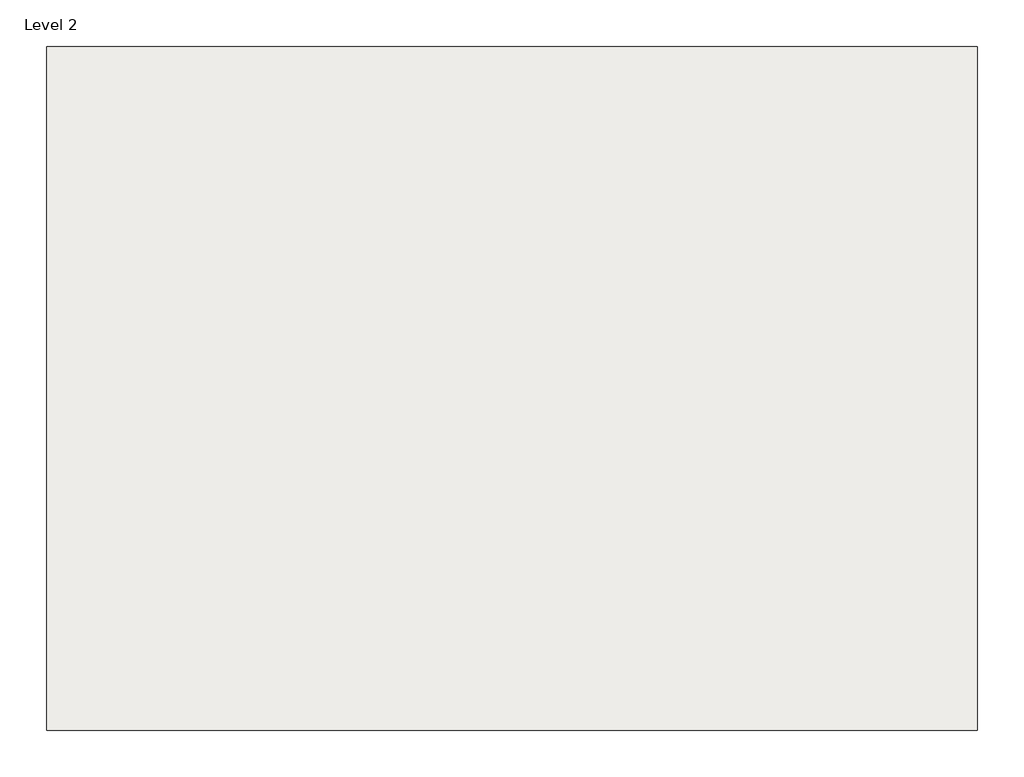
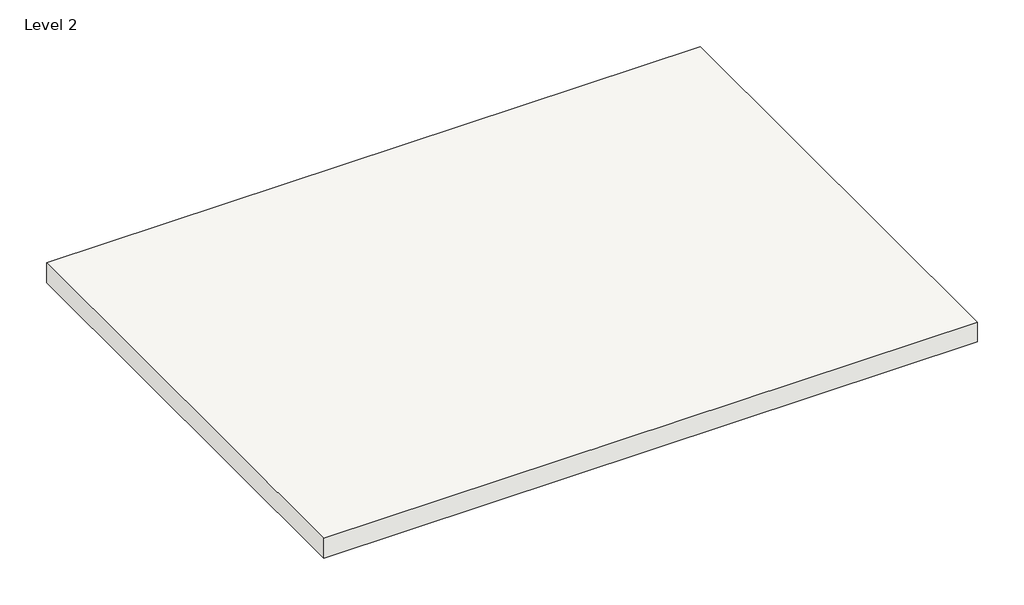
# One storey: 1 roof.
"""IFC4 building model written with IfcOpenShell, lengths in millimetres."""

from ifc_helpers import new_model, si_unit, frame, origin, place, context, project, spatial, polyline, outline, extrude, element, save

model = new_model("IFC4")

# Units and contexts
model_context = context("Model", 3, world=origin())
ifc_project = project(units=[si_unit("LENGTHUNIT", "METRE", prefix="MILLI")], contexts=[model_context])

# Site, building, storey
site = spatial("IfcSite", under=ifc_project)
building = spatial("IfcBuilding", under=site)
storey = spatial("IfcBuildingStorey", under=building, Name="Level 2", Elevation=3048.0)

# Roof
placement = place(None, origin())
element("IfcRoof", 1, ObjectType="Steel Truss - Insulation on Metal Deck - EPDM", at=placement, inside=storey, context=model_context, shape_type="SweptSolid", body=[
    extrude(outline(polyline([(-10694.8266904, 12832.4742707), (6208.8733096, 12832.4742707), (6208.8733096, 411.8742707), (-10694.8266904, 411.8742707), (-10694.8266904, 12832.4742707)])), frame((0.0, 0.0, 3048.0), z_axis=(0.0, 0.0, 1.0), x_axis=(1.0, 0.0, 0.0)), (0.0, 0.0, 1.0), 546.1),
])

save(model, "model.ifc")

# Revit data of these elements
# Type "Steel Truss - Insulation on Metal Deck - EPDM"
#   Assembly Code = "B1020"
#   Layers, outside or top first: 0' - 0 1/4" "Roofing, EPDM Membrane" (function 4); 0' - 5" "Rigid insulation" (function 3); 0' - 0 1/4" "Metal Deck" (function 1); 1' - 4" "Structure, Steel Bar Joist Layer" (function 1)
# Element 1 (IfcRoof, "Steel Truss - Insulation on Metal Deck - EPDM")
#   built-in parameter 1001705 = 11.7917 (stored number, unit not read)
#   built-in parameter 1001710 = 33615
#   Phase Created = New Construction
#   Materials on its faces: "Structure, Steel Bar Joist Layer", "Roofing, EPDM Membrane"
# Materials
#   "Roofing, EPDM Membrane": class "Generic", colour RGB 127 127 127, transparency 0, Description = "EPDM roof membrane", Cost = 0
#   "Rigid insulation": class "Generic", colour RGB 127 127 127, transparency 0, Description = "Rigid foam insulation board", Cost = 0
#   "Metal Deck": class "Metal", colour RGB 199 199 199, transparency 0, Description = "Steel, mill finish", Cost = 0
#   "Structure, Steel Bar Joist Layer": class "Metal", colour RGB 127 127 127, transparency 0, Description = "Bar joists, thermal airspace", Cost = 0
